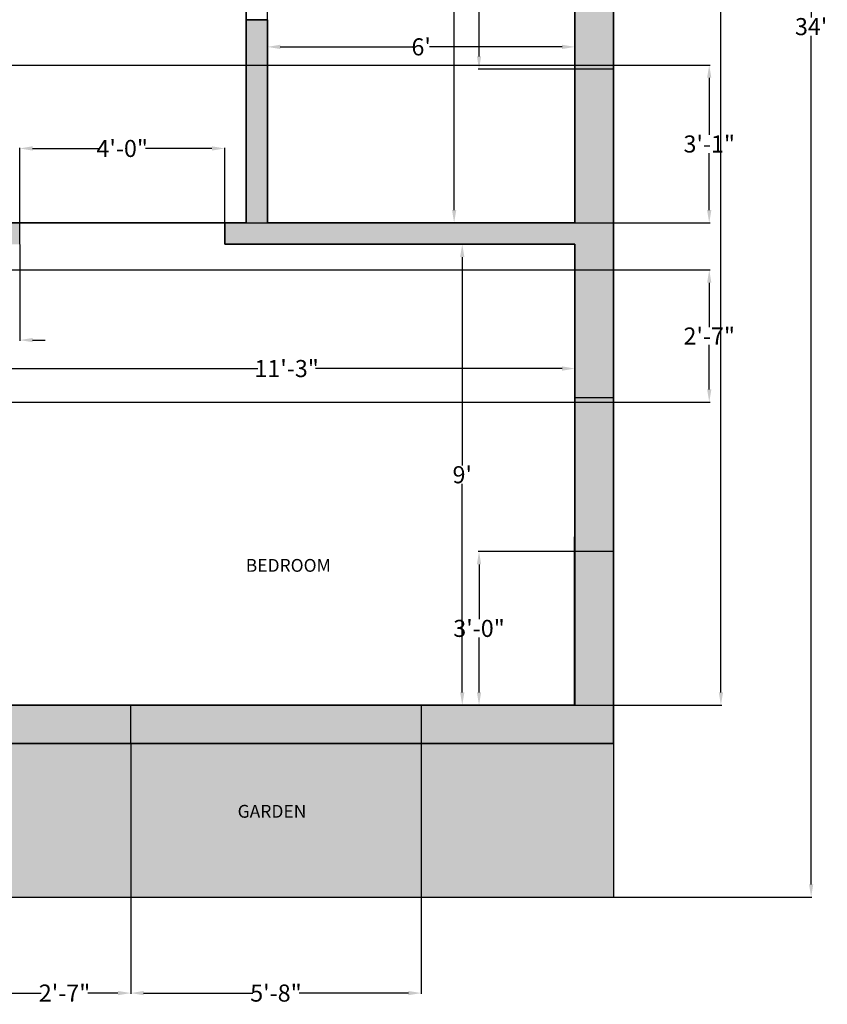
# Model space of a CAD drawing. Units: inches. Extents: x 477 to 929, y 265 to 727.
# Tile 2 of 4: x 740 to 929, y 265 to 496. Entities that reach past the tile are written whole.
import ezdxf

# ---------------------------------------------------------------- set-up
doc = ezdxf.new("R2010")
doc.units = ezdxf.units.IN
doc.header["$MEASUREMENT"] = 0
for name, color, linetype, lineweight, true_color in [('A-ANNO-DIMS', 215, 'Continuous', 18, 0xa953a0), ('A-WALL-PATT', 244, 'Continuous', 13, 0x991b1e), ('L-PLNT-PATT', 114, 'Continuous', 13, 0x139b48)]:
    doc.layers.add(name, color=color, linetype=linetype, lineweight=lineweight, true_color=true_color)
for name, color, linetype, lineweight in [('A-AREA-IDEN', 3, 'Continuous', 25), ('A-GLAZ', 4, 'Continuous', 25), ('A-GLAZ-PATT', 7, 'Continuous', 13), ('A-WALL', 7, 'Continuous', 35), ('L-SITE', 7, 'Continuous', 25)]:
    doc.layers.add(name, color=color, linetype=linetype, lineweight=lineweight)
doc.styles.get("Standard").update_dxf_attribs({"font": 'arial.ttf'})
doc.dimstyles.get("Standard").update_dxf_attribs({"dimtxt": 4, "dimasz": 3, "dimexe": 0.18, "dimexo": 0.0625, "dimgap": 0.09, "dimtad": 0, "dimtih": 1, "dimtoh": 1, "dimdec": 0, "dimzin": 0, "dimdsep": 46, "dimlunit": 3, "dimtxsty": 'Standard', "dimcen": 0, "dimadec": 0, "dimazin": 0, "dimtfac": 1, "dimtdec": 0, "dimtofl": 0, "dimtmove": 0, "dimatfit": 3, "dimfxl": 1, "dimtolj": 1, "dimtzin": 0, "dimarcsym": 1})

# ---------------------------------------------------------------- blocks, each defined once
blk = doc.blocks.new('*D5')
at = {"layer": 'A-ANNO-DIMS', "color": 0, "lineweight": -2, "transparency": 16777216}
for p, q in [((735.33, 335.27), (735.33, 414.27)), ((738.33, 414.09), (796.06, 414.09)), ((867.33, 414.09), (809.61, 414.09)), ((870.33, 335.27), (870.33, 414.27))]:
    blk.add_line(p, q, dxfattribs=at)
at = {"layer": 'A-ANNO-DIMS', "color": 0, "transparency": 16777216}
for points in [[(738.33, 414.59), (738.33, 413.59), (735.33, 414.09)], [(867.33, 414.59), (867.33, 413.59), (870.33, 414.09)]]:
    blk.add_solid(points, dxfattribs=at)
at = {"layer": 'Defpoints', "color": 0, "transparency": 16777216}
for p in [(870.33, 414.09), (735.33, 335.21), (870.33, 335.21)]:
    blk.add_point(p, dxfattribs=at)
at = {"layer": 'A-ANNO-DIMS', "color": 0, "transparency": 16777216, "insert": (802.83, 414.09), "char_height": 4, "attachment_point": 5}
blk.add_mtext('\\A1;11\'-3"', dxfattribs=at)
blk = doc.blocks.new('*D6')
at = {"layer": 'A-ANNO-DIMS', "color": 0, "lineweight": -2, "transparency": 16777216}
for p, q in [((870.27, 443.21), (843.77, 443.21)), ((843.95, 440.21), (843.95, 391.34)), ((843.95, 338.21), (843.95, 387.07)), ((870.27, 335.21), (843.77, 335.21))]:
    blk.add_line(p, q, dxfattribs=at)
at = {"layer": 'A-ANNO-DIMS', "color": 0, "transparency": 16777216}
for points in [[(843.45, 440.21), (844.45, 440.21), (843.95, 443.21)], [(843.45, 338.21), (844.45, 338.21), (843.95, 335.21)]]:
    blk.add_solid(points, dxfattribs=at)
at = {"layer": 'Defpoints', "color": 0, "transparency": 16777216}
for p in [(870.33, 443.21), (843.95, 335.21), (870.33, 335.21)]:
    blk.add_point(p, dxfattribs=at)
at = {"layer": 'A-ANNO-DIMS', "color": 0, "transparency": 16777216, "insert": (843.95, 389.21), "char_height": 4, "attachment_point": 5}
blk.add_mtext("\\A1;9'", dxfattribs=at)
blk = doc.blocks.new('*D7')
at = {"layer": 'A-ANNO-DIMS', "color": 0, "lineweight": -2, "transparency": 16777216}
for p, q in [((870.27, 557.21), (841.87, 557.21)), ((842.05, 554.21), (842.05, 504.84)), ((842.05, 451.21), (842.05, 500.57)), ((870.27, 448.21), (841.87, 448.21))]:
    blk.add_line(p, q, dxfattribs=at)
at = {"layer": 'A-ANNO-DIMS', "color": 0, "transparency": 16777216}
for points in [[(841.55, 554.21), (842.55, 554.21), (842.05, 557.21)], [(841.55, 451.21), (842.55, 451.21), (842.05, 448.21)]]:
    blk.add_solid(points, dxfattribs=at)
at = {"layer": 'Defpoints', "color": 0, "transparency": 16777216}
for p in [(870.33, 557.21), (842.05, 448.21), (870.33, 448.21)]:
    blk.add_point(p, dxfattribs=at)
at = {"layer": 'A-ANNO-DIMS', "color": 0, "transparency": 16777216, "insert": (842.05, 502.71), "char_height": 4, "attachment_point": 5}
blk.add_mtext('\\A1;9\'-1"', dxfattribs=at)
blk = doc.blocks.new('*D8')
at = {"layer": 'A-ANNO-DIMS', "color": 0, "lineweight": -2, "transparency": 16777216}
for p, q in [((798.33, 495.77), (798.33, 489.28)), ((870.33, 495.77), (870.33, 489.28)), ((801.33, 489.46), (832.39, 489.46)), ((867.33, 489.46), (836.28, 489.46))]:
    blk.add_line(p, q, dxfattribs=at)
at = {"layer": 'A-ANNO-DIMS', "color": 0, "transparency": 16777216}
for points in [[(801.33, 489.96), (801.33, 488.96), (798.33, 489.46)], [(867.33, 489.96), (867.33, 488.96), (870.33, 489.46)]]:
    blk.add_solid(points, dxfattribs=at)
at = {"layer": 'Defpoints', "color": 0, "transparency": 16777216}
for p in [(798.33, 495.83), (870.33, 495.83), (870.33, 489.46)]:
    blk.add_point(p, dxfattribs=at)
at = {"layer": 'A-ANNO-DIMS', "color": 0, "transparency": 16777216, "insert": (834.33, 489.46), "char_height": 4, "attachment_point": 5}
blk.add_mtext("\\A1;6'", dxfattribs=at)
blk = doc.blocks.new('*D17')
at = {"layer": 'A-ANNO-DIMS', "color": 0, "lineweight": -2, "transparency": 16777216}
for p, q in [((879.4, 698.21), (925.82, 698.21)), ((925.64, 695.21), (925.64, 496.34)), ((925.64, 293.21), (925.64, 492.07)), ((879.4, 290.21), (925.82, 290.21))]:
    blk.add_line(p, q, dxfattribs=at)
at = {"layer": 'A-ANNO-DIMS', "color": 0, "transparency": 16777216}
for points in [[(925.14, 695.21), (926.14, 695.21), (925.64, 698.21)], [(925.14, 293.21), (926.14, 293.21), (925.64, 290.21)]]:
    blk.add_solid(points, dxfattribs=at)
at = {"layer": 'Defpoints', "color": 0, "transparency": 16777216}
for p in [(879.33, 698.21), (879.33, 290.21), (925.64, 290.21)]:
    blk.add_point(p, dxfattribs=at)
at = {"layer": 'A-ANNO-DIMS', "color": 0, "transparency": 16777216, "insert": (925.64, 494.21), "char_height": 4, "attachment_point": 5}
blk.add_mtext("\\A1;34'", dxfattribs=at)
blk = doc.blocks.new('*D19')
at = {"layer": 'A-ANNO-DIMS', "color": 0, "lineweight": -2, "transparency": 16777216}
for p, q in [((870.4, 689.14), (904.7, 689.14)), ((904.52, 686.14), (904.52, 514.31)), ((904.52, 338.21), (904.52, 510.04)), ((870.33, 335.21), (904.7, 335.21))]:
    blk.add_line(p, q, dxfattribs=at)
at = {"layer": 'A-ANNO-DIMS', "color": 0, "transparency": 16777216}
for points in [[(904.02, 686.14), (905.02, 686.14), (904.52, 689.14)], [(904.02, 338.21), (905.02, 338.21), (904.52, 335.21)]]:
    blk.add_solid(points, dxfattribs=at)
at = {"layer": 'Defpoints', "color": 0, "transparency": 16777216}
for p in [(870.33, 689.14), (870.27, 335.21), (904.52, 335.21)]:
    blk.add_point(p, dxfattribs=at)
at = {"layer": 'A-ANNO-DIMS', "color": 0, "transparency": 16777216, "insert": (904.52, 512.17), "char_height": 4, "attachment_point": 5}
blk.add_mtext('\\A1;29\'-6"', dxfattribs=at)
blk = doc.blocks.new('WIN-JAMBS-36IN')
for p, q in [((9, 36), (0, 36)), ((9, 0), (0, 0))]:
    blk.add_line(p, q)
blk = doc.blocks.new('*D29')
at = {"layer": 'A-ANNO-DIMS', "color": 0, "lineweight": -2, "transparency": 16777216}
for p, q in [((624.43, 485.21), (901.96, 485.21)), ((901.78, 482.21), (901.78, 468.84)), ((901.78, 451.21), (901.78, 464.57)), ((624.43, 448.21), (901.96, 448.21))]:
    blk.add_line(p, q, dxfattribs=at)
at = {"layer": 'A-ANNO-DIMS', "color": 0, "transparency": 16777216}
for points in [[(901.28, 482.21), (902.28, 482.21), (901.78, 485.21)], [(901.28, 451.21), (902.28, 451.21), (901.78, 448.21)]]:
    blk.add_solid(points, dxfattribs=at)
at = {"layer": 'Defpoints', "color": 0, "transparency": 16777216}
for p in [(624.37, 485.21), (901.78, 485.21), (624.37, 448.21)]:
    blk.add_point(p, dxfattribs=at)
at = {"layer": 'A-ANNO-DIMS', "color": 0, "transparency": 16777216, "insert": (901.78, 466.71), "char_height": 4, "attachment_point": 5}
blk.add_mtext('\\A1;3\'-1"', dxfattribs=at)
blk = doc.blocks.new('*D39')
at = {"layer": 'A-ANNO-DIMS', "color": 0, "lineweight": -2, "transparency": 16777216}
for p, q in [((790.33, 720.66), (787.33, 720.66)), ((793.33, 448.27), (793.33, 720.84)), ((798.33, 448.27), (798.33, 720.84)), ((801.33, 720.66), (804.33, 720.66))]:
    blk.add_line(p, q, dxfattribs=at)
at = {"layer": 'A-ANNO-DIMS', "color": 0, "transparency": 16777216}
for points in [[(790.33, 721.16), (790.33, 720.16), (793.33, 720.66)], [(801.33, 721.16), (801.33, 720.16), (798.33, 720.66)]]:
    blk.add_solid(points, dxfattribs=at)
at = {"layer": 'Defpoints', "color": 0, "transparency": 16777216}
for p in [(798.33, 720.66), (793.33, 448.21), (798.33, 448.21)]:
    blk.add_point(p, dxfattribs=at)
at = {"layer": 'A-ANNO-DIMS', "color": 0, "transparency": 16777216, "insert": (809.74, 720.66), "char_height": 4, "attachment_point": 5}
blk.add_mtext('\\A1;0\'-5"', dxfattribs=at)
blk = doc.blocks.new('*D52')
at = {"layer": 'A-ANNO-DIMS', "color": 0, "lineweight": -2, "transparency": 16777216}
for p, q in [((870.27, 521.21), (847.7, 521.21)), ((847.88, 518.21), (847.88, 504.84)), ((847.88, 487.21), (847.88, 500.57)), ((870.27, 484.21), (847.7, 484.21))]:
    blk.add_line(p, q, dxfattribs=at)
at = {"layer": 'A-ANNO-DIMS', "color": 0, "transparency": 16777216}
for points in [[(847.38, 518.21), (848.38, 518.21), (847.88, 521.21)], [(847.38, 487.21), (848.38, 487.21), (847.88, 484.21)]]:
    blk.add_solid(points, dxfattribs=at)
at = {"layer": 'Defpoints', "color": 0, "transparency": 16777216}
for p in [(847.88, 521.21), (870.33, 521.21), (870.33, 484.21)]:
    blk.add_point(p, dxfattribs=at)
at = {"layer": 'A-ANNO-DIMS', "color": 0, "transparency": 16777216, "insert": (847.88, 502.71), "char_height": 4, "attachment_point": 5}
blk.add_mtext('\\A1;3\'-1"', dxfattribs=at)
blk = doc.blocks.new('*D53')
at = {"layer": 'A-ANNO-DIMS', "color": 0, "lineweight": -2, "transparency": 16777216}
for p, q in [((870.27, 371.21), (847.7, 371.21)), ((847.88, 368.21), (847.88, 355.34)), ((847.88, 338.21), (847.88, 351.07)), ((870.27, 335.21), (847.7, 335.21))]:
    blk.add_line(p, q, dxfattribs=at)
at = {"layer": 'A-ANNO-DIMS', "color": 0, "transparency": 16777216}
for points in [[(847.38, 368.21), (848.38, 368.21), (847.88, 371.21)], [(847.38, 338.21), (848.38, 338.21), (847.88, 335.21)]]:
    blk.add_solid(points, dxfattribs=at)
at = {"layer": 'Defpoints', "color": 0, "transparency": 16777216}
for p in [(847.88, 371.21), (870.33, 371.21), (870.33, 335.21)]:
    blk.add_point(p, dxfattribs=at)
at = {"layer": 'A-ANNO-DIMS', "color": 0, "transparency": 16777216, "insert": (847.88, 353.21), "char_height": 4, "attachment_point": 5}
blk.add_mtext('\\A1;3\'-0"', dxfattribs=at)
blk = doc.blocks.new('*D55')
at = {"layer": 'A-ANNO-DIMS', "color": 0, "lineweight": -2, "transparency": 16777216}
for p, q in [((735.33, 326.14), (735.33, 267.58)), ((766.33, 326.14), (766.33, 267.58)), ((738.33, 267.76), (745.39, 267.76)), ((763.33, 267.76), (756.27, 267.76))]:
    blk.add_line(p, q, dxfattribs=at)
at = {"layer": 'A-ANNO-DIMS', "color": 0, "transparency": 16777216}
for points in [[(738.33, 268.26), (738.33, 267.26), (735.33, 267.76)], [(763.33, 268.26), (763.33, 267.26), (766.33, 267.76)]]:
    blk.add_solid(points, dxfattribs=at)
at = {"layer": 'Defpoints', "color": 0, "transparency": 16777216}
for p in [(735.33, 326.21), (766.33, 326.21), (766.33, 267.76)]:
    blk.add_point(p, dxfattribs=at)
at = {"layer": 'A-ANNO-DIMS', "color": 0, "transparency": 16777216, "insert": (750.83, 267.76), "char_height": 4, "attachment_point": 5}
blk.add_mtext('\\A1;2\'-7"', dxfattribs=at)
blk = doc.blocks.new('*D56')
at = {"layer": 'A-ANNO-DIMS', "color": 0, "lineweight": -2, "transparency": 16777216}
for p, q in [((766.33, 326.14), (766.33, 267.58)), ((834.33, 326.14), (834.33, 267.58)), ((769.33, 267.76), (794.93, 267.76)), ((831.33, 267.76), (805.74, 267.76))]:
    blk.add_line(p, q, dxfattribs=at)
at = {"layer": 'A-ANNO-DIMS', "color": 0, "transparency": 16777216}
for points in [[(769.33, 268.26), (769.33, 267.26), (766.33, 267.76)], [(831.33, 268.26), (831.33, 267.26), (834.33, 267.76)]]:
    blk.add_solid(points, dxfattribs=at)
at = {"layer": 'Defpoints', "color": 0, "transparency": 16777216}
for p in [(766.33, 326.21), (834.33, 326.21), (834.33, 267.76)]:
    blk.add_point(p, dxfattribs=at)
at = {"layer": 'A-ANNO-DIMS', "color": 0, "transparency": 16777216, "insert": (800.33, 267.76), "char_height": 4, "attachment_point": 5}
blk.add_mtext('\\A1;5\'-8"', dxfattribs=at)
blk = doc.blocks.new('*D58')
at = {"layer": 'A-ANNO-DIMS', "color": 0, "lineweight": -2, "transparency": 16777216}
for p, q in [((629.4, 437.21), (901.96, 437.21)), ((901.78, 434.21), (901.78, 423.8)), ((901.78, 409.21), (901.78, 419.61)), ((629.4, 406.21), (901.96, 406.21))]:
    blk.add_line(p, q, dxfattribs=at)
at = {"layer": 'A-ANNO-DIMS', "color": 0, "transparency": 16777216}
for points in [[(901.28, 434.21), (902.28, 434.21), (901.78, 437.21)], [(901.28, 409.21), (902.28, 409.21), (901.78, 406.21)]]:
    blk.add_solid(points, dxfattribs=at)
at = {"layer": 'Defpoints', "color": 0, "transparency": 16777216}
for p in [(629.33, 437.21), (901.78, 437.21), (629.33, 406.21)]:
    blk.add_point(p, dxfattribs=at)
at = {"layer": 'A-ANNO-DIMS', "color": 0, "transparency": 16777216, "insert": (901.78, 421.71), "char_height": 4, "attachment_point": 5}
blk.add_mtext('\\A1;2\'-7"', dxfattribs=at)
blk = doc.blocks.new('*D63')
at = {"layer": 'A-ANNO-DIMS', "color": 0, "lineweight": -2, "transparency": 16777216}
for p, q in [((740.33, 443.27), (740.33, 465.84)), ((743.33, 465.66), (758.85, 465.66)), ((785.33, 465.66), (769.82, 465.66)), ((788.33, 443.27), (788.33, 465.84))]:
    blk.add_line(p, q, dxfattribs=at)
at = {"layer": 'A-ANNO-DIMS', "color": 0, "transparency": 16777216}
for points in [[(743.33, 466.16), (743.33, 465.16), (740.33, 465.66)], [(785.33, 466.16), (785.33, 465.16), (788.33, 465.66)]]:
    blk.add_solid(points, dxfattribs=at)
at = {"layer": 'Defpoints', "color": 0, "transparency": 16777216}
for p in [(788.33, 465.66), (740.33, 443.21), (788.33, 443.21)]:
    blk.add_point(p, dxfattribs=at)
at = {"layer": 'A-ANNO-DIMS', "color": 0, "transparency": 16777216, "insert": (764.33, 465.66), "char_height": 4, "attachment_point": 5}
blk.add_mtext('\\A1;4\'-0"', dxfattribs=at)
blk = doc.blocks.new('*D65')
at = {"layer": 'A-ANNO-DIMS', "color": 0, "lineweight": -2, "transparency": 16777216}
for p, q in [((735.33, 443.14), (735.33, 420.58)), ((740.33, 443.14), (740.33, 420.58)), ((732.33, 420.76), (729.33, 420.76)), ((743.33, 420.76), (746.33, 420.76))]:
    blk.add_line(p, q, dxfattribs=at)
at = {"layer": 'A-ANNO-DIMS', "color": 0, "transparency": 16777216}
for points in [[(732.33, 421.26), (732.33, 420.26), (735.33, 420.76)], [(743.33, 421.26), (743.33, 420.26), (740.33, 420.76)]]:
    blk.add_solid(points, dxfattribs=at)
at = {"layer": 'Defpoints', "color": 0, "transparency": 16777216}
for p in [(735.33, 443.21), (740.33, 443.21), (735.33, 420.76)]:
    blk.add_point(p, dxfattribs=at)
at = {"layer": 'A-ANNO-DIMS', "color": 0, "transparency": 16777216, "insert": (723.93, 420.76), "char_height": 4, "attachment_point": 5}
blk.add_mtext('\\A1;0\'-5"', dxfattribs=at)

msp = doc.modelspace()

# ---------------------------------------------------------------- hatches: boundary and pattern name
at = {"layer": 'A-GLAZ-PATT'}
h = msp.add_hatch(color=256, dxfattribs=at)
h.dxf.hatch_style = 1
h.paths.add_polyline_path([(588.33, 698.21), (552.33, 698.21), (552.33, 689.21), (588.33, 689.21)])
h.paths.add_polyline_path([(659.33, 698.21), (647.33, 698.21), (647.33, 689.21), (659.33, 689.21)])
h.paths.add_polyline_path([(712.33, 698.21), (700.33, 698.21), (700.33, 689.21), (712.33, 689.21)])
h.paths.add_polyline_path([(834.33, 698.21), (771.33, 698.21), (771.33, 689.21), (834.33, 689.21)])
h.paths.add_polyline_path([(879.33, 653.21), (870.33, 653.21), (870.33, 598.21), (879.33, 598.21)])
h.paths.add_polyline_path([(879.33, 521.21), (870.33, 521.21), (870.33, 484.21), (879.33, 484.21)])
h.paths.add_polyline_path([(879.33, 407.21), (870.33, 407.21), (870.33, 371.21), (879.33, 371.21)])
h.paths.add_polyline_path([(834.33, 335.21), (766.33, 335.21), (766.33, 326.21), (834.33, 326.21)])
h.paths.add_polyline_path([(588.33, 335.21), (552.33, 335.21), (552.33, 326.21), (588.33, 326.21)])
h.paths.add_polyline_path([(516.33, 430.21), (507.33, 430.21), (507.33, 371.21), (516.33, 371.21)])
h.paths.add_polyline_path([(516.33, 539.21), (507.33, 539.21), (507.33, 466.21), (516.33, 466.21)])
h.paths.add_polyline_path([(516.33, 653.21), (507.33, 653.21), (507.33, 598.21), (516.33, 598.21)])
at = {"layer": 'A-WALL-PATT'}
h = msp.add_hatch(color=256, dxfattribs=at)
h.dxf.hatch_style = 1
h.paths.add_polyline_path([(516.33, 598.21), (507.33, 598.21), (507.33, 539.21), (516.33, 539.21), (516.33, 557.21), (570.33, 557.21), (570.33, 562.21), (516.33, 562.21)])
h.paths.add_polyline_path([(552.33, 698.21), (507.33, 698.21), (507.33, 653.21), (516.33, 653.21), (516.33, 689.21), (552.33, 689.21)])
h.paths.add_polyline_path([(647.33, 698.21), (588.33, 698.21), (588.33, 689.21), (647.33, 689.21)])
h.paths.add_polyline_path([(700.33, 698.21), (659.33, 698.21), (659.33, 689.21), (700.33, 689.21)])
h.paths.add_polyline_path([(771.33, 698.21), (712.33, 698.21), (712.33, 689.21), (771.33, 689.21)])
h.paths.add_polyline_path([(879.33, 698.21), (834.33, 698.21), (834.33, 689.21), (870.33, 689.21), (870.33, 653.21), (879.33, 653.21)])
h.paths.add_polyline_path([(879.33, 598.21), (870.33, 598.21), (870.33, 562.21), (735.33, 562.21), (735.33, 568.21), (730.33, 568.21), (730.33, 557.21), (793.33, 557.21), (793.33, 551.21), (798.33, 551.21), (798.33, 557.21), (870.33, 557.21), (870.33, 521.21), (879.33, 521.21)])
h.paths.add_polyline_path([(879.33, 484.21), (870.33, 484.21), (870.33, 448.21), (798.33, 448.21), (798.33, 495.83), (793.33, 495.83), (793.33, 448.21), (788.33, 448.21), (788.33, 443.21), (870.33, 443.21), (870.33, 407.21), (879.33, 407.21)])
h.paths.add_polyline_path([(735.33, 443.21), (740.33, 443.21), (740.33, 448.21), (730.33, 448.21), (730.33, 400.21), (682.33, 400.21), (682.33, 395.21), (730.33, 395.21), (730.33, 326.21), (766.33, 326.21), (766.33, 335.21), (735.33, 335.21)])
h.paths.add_polyline_path([(879.33, 371.21), (870.33, 371.21), (870.33, 335.21), (834.33, 335.21), (834.33, 326.21), (879.33, 326.21)])
h.paths.add_polyline_path([(516.33, 466.21), (507.33, 466.21), (507.33, 430.21), (516.33, 430.21), (516.33, 443.21), (624.33, 443.21), (624.33, 437.21), (629.33, 437.21), (629.33, 448.21), (516.33, 448.21)])
h.paths.add_polyline_path([(629.33, 600.21), (700.33, 600.21), (700.33, 605.21), (682.33, 605.21), (682.33, 689.21), (677.33, 689.21), (677.33, 605.21), (629.33, 605.21), (629.33, 611.21), (624.33, 611.21), (624.33, 562.21), (618.33, 562.21), (618.33, 557.21), (629.33, 557.21)])
h.paths.add_polyline_path([(629.33, 689.21), (624.33, 689.21), (624.33, 653.21), (629.33, 653.21)], flags=17)
at = {"layer": 'L-PLNT-PATT'}
h = msp.add_hatch(dxfattribs=at)
h.set_pattern_fill('GRASS', color=256, scale=5)
h.paths.add_polyline_path([(624.33, 326.21), (507.33, 326.21), (507.33, 290.21), (624.33, 290.21)])
h.paths.add_polyline_path([(879.33, 326.21), (735.33, 326.21), (735.33, 290.21), (879.33, 290.21)])
h.paths.add_polyline_path([(790.59, 308.02), (810.07, 308.02), (810.07, 312.68), (790.59, 312.68)], flags=24)

# ---------------------------------------------------------------- linework, layer by layer
at = {"layer": 'A-GLAZ'}
for p, q in [((879.33, 484.21), (870.33, 484.21)), ((766.33, 326.21), (766.33, 335.21)), ((834.33, 335.21), (834.33, 326.21))]:
    msp.add_line(p, q, dxfattribs=at)
at = {"layer": 'A-WALL'}
for p, q in [((879.33, 698.21), (879.33, 326.21)), ((879.33, 698.21), (879.33, 326.21)), ((870.33, 689.21), (870.33, 448.21)), ((793.33, 557.21), (793.33, 448.21)), ((870.33, 557.21), (870.33, 448.21)), ((798.33, 495.83), (793.33, 495.83)), ((798.33, 495.83), (798.33, 448.21)), ((798.33, 489.28), (798.33, 495.83)), ((793.33, 448.21), (730.33, 448.21)), ((788.33, 448.21), (788.33, 443.21)), ((870.33, 448.21), (798.33, 448.21)), ((842.05, 448.21), (870.27, 448.21)), ((870.33, 443.21), (788.33, 443.21)), ((843.95, 443.21), (870.33, 443.21)), ((870.33, 443.21), (870.33, 335.21)), ((870.27, 335.21), (870.33, 414.27)), ((870.33, 335.21), (735.33, 335.21)), ((870.27, 335.21), (843.95, 335.21)), ((507.33, 326.21), (879.33, 326.21))]:
    msp.add_line(p, q, dxfattribs=at)
at = {"layer": 'L-SITE'}
for p in [(879.33, 326.21), (507.33, 290.21)]:
    msp.add_line(p, (879.33, 290.21), dxfattribs=at)

# ---------------------------------------------------------------- block references
at = {"layer": 'A-GLAZ'}
msp.add_blockref('WIN-JAMBS-36IN', (870.33, 371.21), dxfattribs=at)

# ---------------------------------------------------------------- texts
at = {"layer": 'A-AREA-IDEN'}
msp.add_text('GARDEN', height=3, dxfattribs=at).set_placement((791.36, 308.85))
at = {"layer": 'A-AREA-IDEN', "insert": (793.26, 369.47), "char_height": 3, "attachment_point": 1}
msp.add_mtext_dynamic_manual_height_columns('BEDROOM', width=70.7384, gutter_width=1, heights=[0], dxfattribs=at)

# ---------------------------------------------------------------- dimensions: what is measured, and where the dimension line sits
at = {"layer": 'A-ANNO-DIMS'}
for base, p1, p2, override, picture, middle in [((798.33, 720.66), (793.33, 448.21), (798.33, 448.21), {"dimdec": 1, "dimlfac": 1, "dimrnd": 0, "dimzin": 1, "dimdsep": 46, "dimlunit": 4, "dimfrac": 2}, '*D39', (809.74, 720.66)), ((870.33, 489.46), (798.33, 495.83), (870.33, 495.83), {"dimclrd": 0, "dimclre": 0, "dimclrt": 0}, '*D8', (834.33, 489.46)), ((788.33, 465.66), (740.33, 443.21), (788.33, 443.21), {"dimdec": 1, "dimlfac": 1, "dimrnd": 0, "dimzin": 1, "dimdsep": 46, "dimlunit": 4, "dimfrac": 2}, '*D63', (764.33, 465.66)), ((870.33, 414.09), (735.33, 335.21), (870.33, 335.21), {"dimclrd": 0, "dimclre": 0, "dimclrt": 0}, '*D5', (802.83, 414.09)), ((766.33, 267.76), (735.33, 326.21), (766.33, 326.21), {"dimdec": 1, "dimlfac": 1, "dimrnd": 0, "dimzin": 1, "dimdsep": 46, "dimlunit": 4, "dimfrac": 2}, '*D55', (750.83, 267.76)), ((834.33, 267.76), (766.33, 326.21), (834.33, 326.21), {"dimdec": 1, "dimlfac": 1, "dimrnd": 0, "dimzin": 1, "dimdsep": 46, "dimlunit": 4, "dimfrac": 2}, '*D56', (800.33, 267.76))]:
    dim = msp.add_linear_dim(base=base, p1=p1, p2=p2, dimstyle='Standard', override=override, dxfattribs=at)
    dim.commit()
    dim.dimension.update_dxf_attribs({"geometry": picture, "text_midpoint": middle})
for base, p1, p2, angle, override, picture, middle in [((925.64, 290.21), (879.33, 698.21), (879.33, 290.21), 90, {"dimclrd": 0, "dimclre": 0, "dimclrt": 0}, '*D17', (925.64, 494.21)), ((904.52, 335.21), (870.33, 689.14), (870.27, 335.21), 90, {"dimclrd": 0, "dimclre": 0, "dimclrt": 0}, '*D19', (904.52, 512.17)), ((842.05, 448.21), (870.33, 557.21), (870.33, 448.21), 90, {"dimclrd": 0, "dimclre": 0, "dimclrt": 0}, '*D7', (842.05, 502.71)), ((847.88, 521.21), (870.33, 484.21), (870.33, 521.21), 90, {"dimdec": 1, "dimlfac": 1, "dimrnd": 0, "dimzin": 1, "dimdsep": 46, "dimlunit": 4, "dimfrac": 2}, '*D52', (847.88, 502.71)), ((901.78, 485.21), (624.37, 448.21), (624.37, 485.21), 90, {"dimdec": 1, "dimlfac": 1, "dimrnd": 0, "dimzin": 1, "dimdsep": 46, "dimlunit": 4, "dimfrac": 2}, '*D29', (901.78, 466.71)), ((735.33, 420.76), (740.33, 443.21), (735.33, 443.21), 180, {"dimdec": 1, "dimlfac": 1, "dimrnd": 0, "dimzin": 1, "dimdsep": 46, "dimlunit": 4, "dimfrac": 2}, '*D65', (723.93, 420.76)), ((843.95, 335.21), (870.33, 443.21), (870.33, 335.21), 90, {"dimclrd": 0, "dimclre": 0, "dimclrt": 0}, '*D6', (843.95, 389.21)), ((901.78, 437.21), (629.33, 406.21), (629.33, 437.21), 90, {"dimdec": 1, "dimlfac": 1, "dimrnd": 0, "dimzin": 1, "dimdsep": 46, "dimlunit": 4, "dimfrac": 2}, '*D58', (901.78, 421.71)), ((847.88, 371.21), (870.33, 335.21), (870.33, 371.21), 90, {"dimdec": 1, "dimlfac": 1, "dimrnd": 0, "dimzin": 1, "dimdsep": 46, "dimlunit": 4, "dimfrac": 2}, '*D53', (847.88, 353.21))]:
    dim = msp.add_linear_dim(base=base, p1=p1, p2=p2, angle=angle, dimstyle='Standard', override=override, dxfattribs=at)
    dim.commit()
    dim.dimension.update_dxf_attribs({"geometry": picture, "text_midpoint": middle})

doc.saveas('drawing.dxf')
